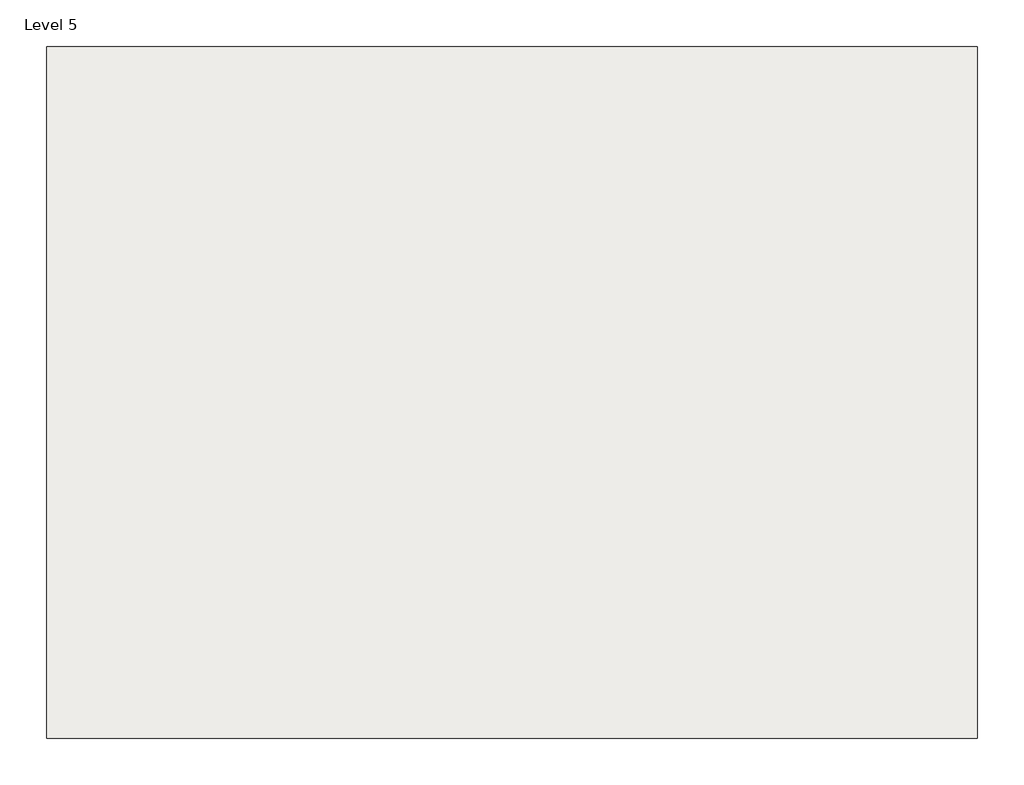
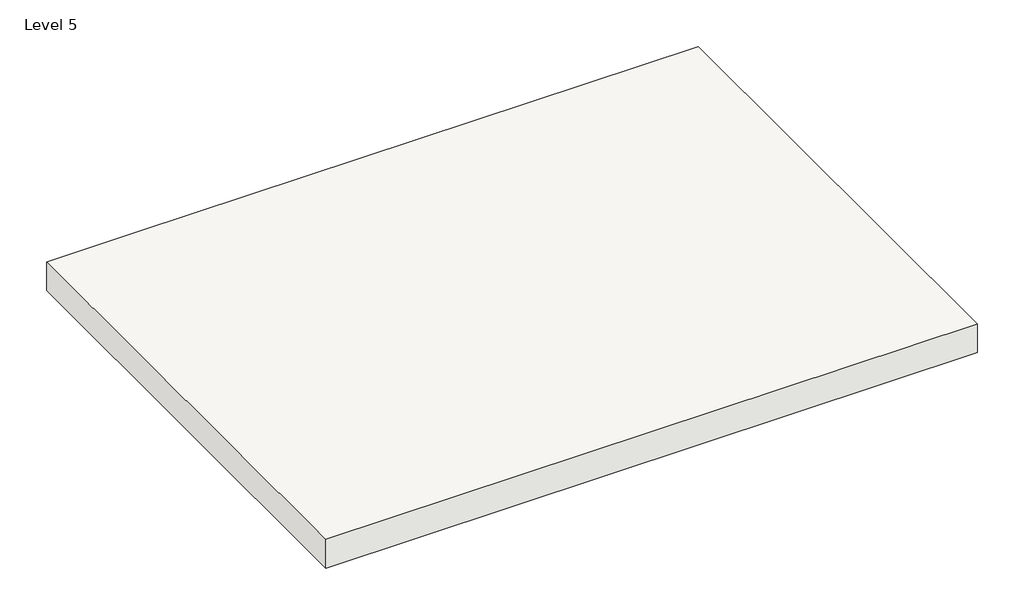
# One storey: 1 roof.
"""IFC4 building model written with IfcOpenShell, lengths in millimetres."""

from ifc_helpers import new_model, si_unit, frame, origin, place, context, project, spatial, polyline, outline, extrude, element, save

model = new_model("IFC4")

# Units and contexts
model_context = context("Model", 3, world=origin())
ifc_project = project(units=[si_unit("LENGTHUNIT", "METRE", prefix="MILLI")], contexts=[model_context])

# Site, building, storey
site = spatial("IfcSite", under=ifc_project)
building = spatial("IfcBuilding", under=site)
storey = spatial("IfcBuildingStorey", under=building, Name="Level 5", Elevation=14630.4)

# Roof
placement = place(None, origin())
element("IfcRoof", 1, ObjectType="Generic - 12\"", at=placement, inside=storey, context=model_context, shape_type="SweptSolid", body=[
    extrude(outline(polyline([(-10924.0857575, 5703.7959854), (-10018.4747472, 5703.7959854), (-4379.6747472, 5703.7959854), (-4379.6747472, 842.4609482), (-10924.0857575, 842.4609482), (-10924.0857575, 5703.7959854)])), frame((0.0, 0.0, 14630.4), z_axis=(0.0, 0.0, 1.0), x_axis=(1.0, 0.0, 0.0)), (0.0, 0.0, 1.0), 304.8),
])

save(model, "model.ifc")

# Revit data of these elements
# Type "Generic - 12\""
#   Assembly Code = "B1020"
#   Layers, outside or top first: 1' - 0" no material (function 1)
# Element 1 (IfcRoof, "Generic - 12\"")
#   built-in parameter 1001705 = 49 (stored number, unit not read)
#   built-in parameter 1001710 = 33615
#   Phase Created = New Construction
#   Materials on its faces: "Default Roof"
# Materials
#   "Default Roof": colour RGB 88 101 114, transparency 0
